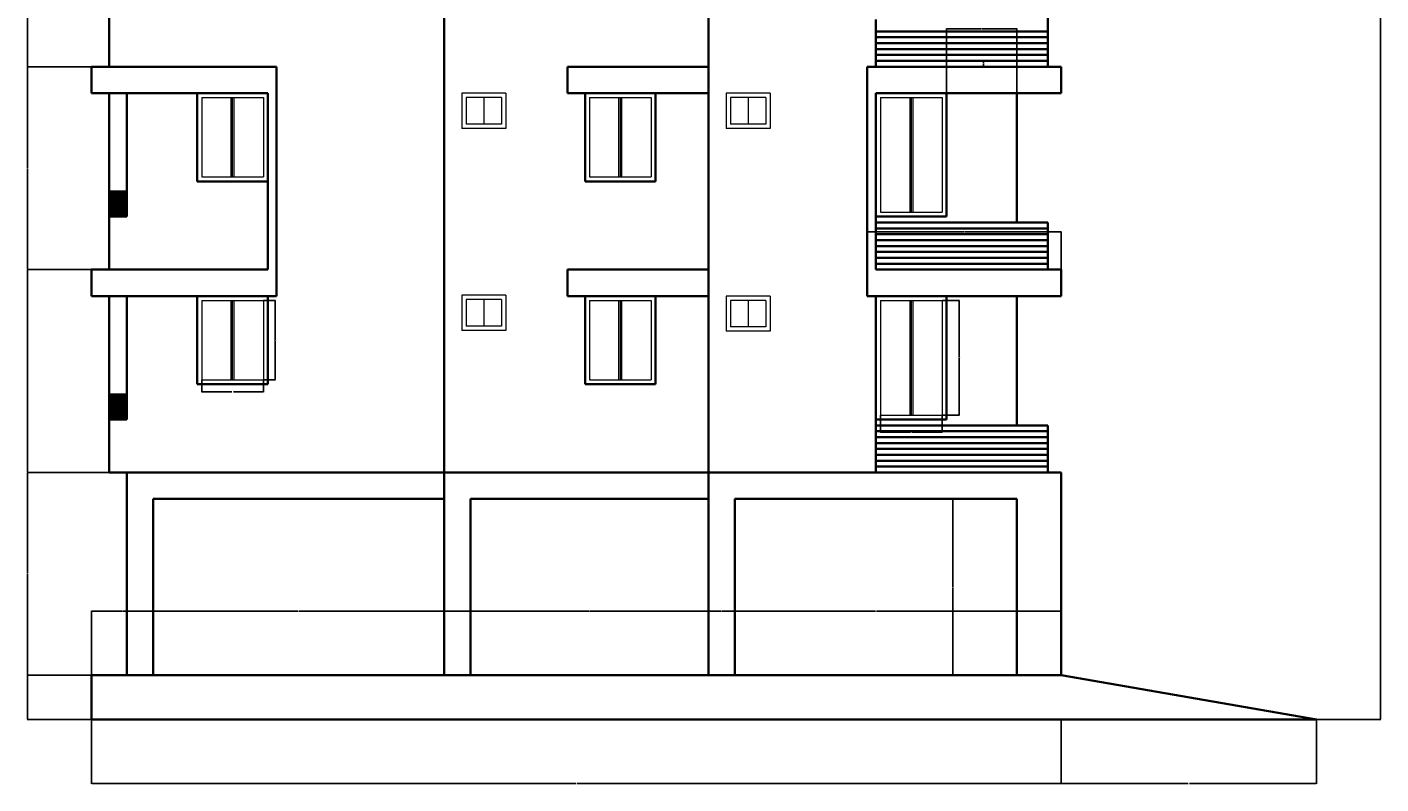
# Model space of a CAD drawing. Units: inches. Extents: x 2136 to 3058, y 322 to 1274.
# Tile 1 of 3: x 2136 to 3058, y 322 to 837. Entities that reach past the tile are written whole.
import ezdxf

# ---------------------------------------------------------------- set-up
doc = ezdxf.new("R2010")
doc.units = ezdxf.units.IN
for name, color, linetype, lineweight in [('A-ANNO-DIMS', 2, 'Continuous', 18), ('A-ELEV', 7, 'Continuous', 35), ('A-GLAZ', 4, 'Continuous', 18)]:
    doc.layers.add(name, color=color, linetype=linetype, lineweight=lineweight)
doc.styles.get("Standard").update_dxf_attribs({"font": 'arial.ttf'})
doc.dimstyles.get("Standard").update_dxf_attribs({"dimtxt": 0.18, "dimasz": 0.18, "dimexe": 0.18, "dimexo": 0.0625, "dimgap": 0.09, "dimtad": 0, "dimtih": 1, "dimtoh": 1, "dimdec": 4, "dimzin": 0, "dimdsep": 46, "dimtxsty": 'Standard', "dimcen": 0.09, "dimadec": 0, "dimazin": 0, "dimtfac": 1, "dimtdec": 4, "dimtofl": 0, "dimtmove": 0, "dimatfit": 3, "dimfxl": 1, "dimtolj": 1, "dimtzin": 0, "dimarcsym": 0})

# ---------------------------------------------------------------- blocks, each defined once
blk = doc.blocks.new('WIN-SMALL')
for p, q in [((2458.76, 1064.68), (2434.76, 1064.68)), ((2434.76, 1064.68), (2434.76, 1046.68)), ((2446.76, 1064.68), (2446.76, 1046.68)), ((2458.76, 1064.68), (2458.76, 1046.68)), ((2458.76, 1046.68), (2434.76, 1046.68))]:
    blk.add_line(p, q)
blk = doc.blocks.new('WIN-1200')
for p, q in [((2254.76, 650.67), (2254.76, 596.67)), ((2254.76, 650.67), (2296.76, 650.67)), ((2274.76, 596.67), (2274.76, 650.67)), ((2275.76, 596.67), (2275.76, 650.67)), ((2276.76, 596.67), (2276.76, 650.67)), ((2296.76, 650.67), (2296.76, 596.67)), ((2254.76, 596.67), (2296.76, 596.67))]:
    blk.add_line(p, q)
blk = doc.blocks.new('WIN-TALL')
for p, q in [((2716.76, 650.68), (2716.76, 572.68)), ((2716.76, 650.68), (2758.76, 650.68)), ((2736.76, 650.68), (2736.76, 572.68)), ((2737.76, 650.68), (2737.76, 572.68)), ((2738.76, 650.68), (2738.76, 572.68)), ((2758.76, 650.68), (2758.76, 572.68)), ((2716.76, 572.68), (2758.76, 572.68))]:
    blk.add_line(p, q)
blk = doc.blocks.new('*D6')
at = {"layer": 'A-ANNO-DIMS', "color": 0, "lineweight": -2, "transparency": 16777216}
for p, q in [((2296.82, 650.67), (2305.04, 650.67)), ((2304.86, 650.49), (2304.86, 623.86)), ((2304.86, 596.85), (2304.86, 623.49)), ((2296.82, 596.67), (2305.04, 596.67))]:
    blk.add_line(p, q, dxfattribs=at)
at = {"layer": 'A-ANNO-DIMS', "color": 0, "transparency": 16777216}
for points in [[(2304.83, 650.49), (2304.89, 650.49), (2304.86, 650.67)], [(2304.83, 596.85), (2304.89, 596.85), (2304.86, 596.67)]]:
    blk.add_solid(points, dxfattribs=at)
at = {"layer": 'Defpoints', "color": 0, "transparency": 16777216}
for p in [(2296.76, 650.67), (2304.86, 650.67), (2296.76, 596.67)]:
    blk.add_point(p, dxfattribs=at)
at = {"layer": 'A-ANNO-DIMS', "color": 0, "transparency": 16777216, "insert": (2304.86, 623.67), "char_height": 0.18, "attachment_point": 5}
blk.add_mtext('\\A1;WINDOW W1 54 TYP.', dxfattribs=at)
blk = doc.blocks.new('*D7')
at = {"layer": 'A-ANNO-DIMS', "color": 0, "lineweight": -2, "transparency": 16777216}
for p, q in [((2254.76, 596.61), (2254.76, 588.39)), ((2296.76, 596.61), (2296.76, 588.39)), ((2254.94, 588.57), (2275.23, 588.57)), ((2296.58, 588.57), (2276.29, 588.57))]:
    blk.add_line(p, q, dxfattribs=at)
at = {"layer": 'A-ANNO-DIMS', "color": 0, "transparency": 16777216}
for points in [[(2254.94, 588.6), (2254.94, 588.54), (2254.76, 588.57)], [(2296.58, 588.6), (2296.58, 588.54), (2296.76, 588.57)]]:
    blk.add_solid(points, dxfattribs=at)
at = {"layer": 'Defpoints', "color": 0, "transparency": 16777216}
for p in [(2254.76, 596.67), (2296.76, 596.67), (2296.76, 588.57)]:
    blk.add_point(p, dxfattribs=at)
at = {"layer": 'A-ANNO-DIMS', "color": 0, "transparency": 16777216, "insert": (2275.76, 588.57), "char_height": 0.18, "attachment_point": 5}
blk.add_mtext('\\A1;42 TYP.', dxfattribs=at)
blk = doc.blocks.new('*D8')
at = {"layer": 'A-ANNO-DIMS', "color": 0, "lineweight": -2, "transparency": 16777216}
for p, q in [((2758.82, 650.68), (2770.64, 650.68)), ((2770.46, 650.5), (2770.46, 611.87)), ((2770.46, 572.86), (2770.46, 611.5)), ((2758.82, 572.68), (2770.64, 572.68))]:
    blk.add_line(p, q, dxfattribs=at)
at = {"layer": 'A-ANNO-DIMS', "color": 0, "transparency": 16777216}
for points in [[(2770.43, 650.5), (2770.49, 650.5), (2770.46, 650.68)], [(2770.43, 572.86), (2770.49, 572.86), (2770.46, 572.68)]]:
    blk.add_solid(points, dxfattribs=at)
at = {"layer": 'Defpoints', "color": 0, "transparency": 16777216}
for p in [(2758.76, 650.68), (2770.46, 650.68), (2758.76, 572.68)]:
    blk.add_point(p, dxfattribs=at)
at = {"layer": 'A-ANNO-DIMS', "color": 0, "transparency": 16777216, "insert": (2770.46, 611.68), "char_height": 0.18, "attachment_point": 5}
blk.add_mtext('\\A1;FRENCH WINDOW W3 78 TYP.', dxfattribs=at)
blk = doc.blocks.new('*D9')
at = {"layer": 'A-ANNO-DIMS', "color": 0, "lineweight": -2, "transparency": 16777216}
for p, q in [((2716.76, 572.62), (2716.76, 560.8)), ((2758.76, 572.62), (2758.76, 560.8)), ((2716.94, 560.98), (2737.23, 560.98)), ((2758.58, 560.98), (2738.29, 560.98))]:
    blk.add_line(p, q, dxfattribs=at)
at = {"layer": 'A-ANNO-DIMS', "color": 0, "transparency": 16777216}
for points in [[(2716.94, 561.01), (2716.94, 560.95), (2716.76, 560.98)], [(2758.58, 561.01), (2758.58, 560.95), (2758.76, 560.98)]]:
    blk.add_solid(points, dxfattribs=at)
at = {"layer": 'Defpoints', "color": 0, "transparency": 16777216}
for p in [(2716.76, 572.68), (2758.76, 572.68), (2758.76, 560.98)]:
    blk.add_point(p, dxfattribs=at)
at = {"layer": 'A-ANNO-DIMS', "color": 0, "transparency": 16777216, "insert": (2737.76, 560.98), "char_height": 0.18, "attachment_point": 5}
blk.add_mtext('\\A1;42 TYP.', dxfattribs=at)
blk = doc.blocks.new('*D10')
at = {"layer": 'A-ANNO-DIMS', "color": 0, "lineweight": -2, "transparency": 16777216}
for p, q in [((2179.76, 365.62), (2179.76, 321.8)), ((2839.76, 365.62), (2839.76, 321.8)), ((2179.94, 321.98), (2509.47, 321.98)), ((2839.58, 321.98), (2510.05, 321.98))]:
    blk.add_line(p, q, dxfattribs=at)
at = {"layer": 'A-ANNO-DIMS', "color": 0, "transparency": 16777216}
for points in [[(2179.94, 322.01), (2179.94, 321.95), (2179.76, 321.98)], [(2839.58, 322.01), (2839.58, 321.95), (2839.76, 321.98)]]:
    blk.add_solid(points, dxfattribs=at)
at = {"layer": 'Defpoints', "color": 0, "transparency": 16777216}
for p in [(2179.76, 365.68), (2839.76, 365.68), (2839.76, 321.98)]:
    blk.add_point(p, dxfattribs=at)
at = {"layer": 'A-ANNO-DIMS', "color": 0, "transparency": 16777216, "insert": (2509.76, 321.98), "char_height": 0.18, "attachment_point": 5}
blk.add_mtext('\\A1;660', dxfattribs=at)
blk = doc.blocks.new('*D11')
at = {"layer": 'A-ANNO-DIMS', "color": 0, "lineweight": -2, "transparency": 16777216}
for p, q in [((2839.76, 365.62), (2839.76, 321.8)), ((3013.64, 365.62), (3013.64, 321.8)), ((2839.94, 321.98), (2926.24, 321.98)), ((3013.46, 321.98), (2927.16, 321.98))]:
    blk.add_line(p, q, dxfattribs=at)
at = {"layer": 'A-ANNO-DIMS', "color": 0, "transparency": 16777216}
for points in [[(2839.94, 322.01), (2839.94, 321.95), (2839.76, 321.98)], [(3013.46, 322.01), (3013.46, 321.95), (3013.64, 321.98)]]:
    blk.add_solid(points, dxfattribs=at)
at = {"layer": 'Defpoints', "color": 0, "transparency": 16777216}
for p in [(2839.76, 365.68), (3013.64, 365.68), (3013.64, 321.98)]:
    blk.add_point(p, dxfattribs=at)
at = {"layer": 'A-ANNO-DIMS', "color": 0, "transparency": 16777216, "insert": (2926.7, 321.98), "char_height": 0.18, "attachment_point": 5}
blk.add_mtext('\\A1;173.88', dxfattribs=at)
blk = doc.blocks.new('*D12')
at = {"layer": 'A-ANNO-DIMS', "color": 0, "lineweight": -2, "transparency": 16777216}
for p, q in [((2830.82, 1229.68), (3057.52, 1229.68)), ((3057.34, 1229.5), (3057.34, 797.87)), ((3057.34, 365.86), (3057.34, 797.5)), ((2839.82, 365.68), (3057.52, 365.68))]:
    blk.add_line(p, q, dxfattribs=at)
at = {"layer": 'A-ANNO-DIMS', "color": 0, "transparency": 16777216}
for points in [[(3057.31, 1229.5), (3057.37, 1229.5), (3057.34, 1229.68)], [(3057.31, 365.86), (3057.37, 365.86), (3057.34, 365.68)]]:
    blk.add_solid(points, dxfattribs=at)
at = {"layer": 'Defpoints', "color": 0, "transparency": 16777216}
for p in [(2830.76, 1229.68), (3057.34, 1229.68), (2839.76, 365.68)]:
    blk.add_point(p, dxfattribs=at)
at = {"layer": 'A-ANNO-DIMS', "color": 0, "transparency": 16777216, "insert": (3057.34, 797.68), "char_height": 0.18, "attachment_point": 5}
blk.add_mtext('\\A1;864', dxfattribs=at)
blk = doc.blocks.new('*D13')
at = {"layer": 'A-ANNO-DIMS', "color": 0, "lineweight": -2, "transparency": 16777216}
for p, q in [((2179.7, 395.68), (2135.88, 395.68)), ((2136.06, 395.5), (2136.06, 380.87)), ((2136.06, 365.86), (2136.06, 380.5)), ((2179.7, 365.68), (2135.88, 365.68))]:
    blk.add_line(p, q, dxfattribs=at)
at = {"layer": 'A-ANNO-DIMS', "color": 0, "transparency": 16777216}
for points in [[(2136.03, 395.5), (2136.09, 395.5), (2136.06, 395.68)], [(2136.03, 365.86), (2136.09, 365.86), (2136.06, 365.68)]]:
    blk.add_solid(points, dxfattribs=at)
at = {"layer": 'Defpoints', "color": 0, "transparency": 16777216}
for p in [(2136.06, 395.68), (2179.76, 395.68), (2179.76, 365.68)]:
    blk.add_point(p, dxfattribs=at)
at = {"layer": 'A-ANNO-DIMS', "color": 0, "transparency": 16777216, "insert": (2136.06, 380.68), "char_height": 0.18, "attachment_point": 5}
blk.add_mtext('\\A1;30', dxfattribs=at)
blk = doc.blocks.new('*D14')
at = {"layer": 'A-ANNO-DIMS', "color": 0, "lineweight": -2, "transparency": 16777216}
for p, q in [((2191.7, 533.68), (2135.88, 533.68)), ((2136.06, 533.5), (2136.06, 464.87)), ((2136.06, 395.86), (2136.06, 464.5)), ((2179.7, 395.68), (2135.88, 395.68))]:
    blk.add_line(p, q, dxfattribs=at)
at = {"layer": 'A-ANNO-DIMS', "color": 0, "transparency": 16777216}
for points in [[(2136.03, 533.5), (2136.09, 533.5), (2136.06, 533.68)], [(2136.03, 395.86), (2136.09, 395.86), (2136.06, 395.68)]]:
    blk.add_solid(points, dxfattribs=at)
at = {"layer": 'Defpoints', "color": 0, "transparency": 16777216}
for p in [(2136.06, 533.68), (2191.76, 533.68), (2179.76, 395.68)]:
    blk.add_point(p, dxfattribs=at)
at = {"layer": 'A-ANNO-DIMS', "color": 0, "transparency": 16777216, "insert": (2136.06, 464.68), "char_height": 0.18, "attachment_point": 5}
blk.add_mtext('\\A1;138', dxfattribs=at)
blk = doc.blocks.new('*D15')
at = {"layer": 'A-ANNO-DIMS', "color": 0, "lineweight": -2, "transparency": 16777216}
for p, q in [((2179.7, 671.68), (2135.88, 671.68)), ((2136.06, 671.5), (2136.06, 602.87)), ((2136.06, 533.86), (2136.06, 602.5)), ((2191.7, 533.68), (2135.88, 533.68))]:
    blk.add_line(p, q, dxfattribs=at)
at = {"layer": 'A-ANNO-DIMS', "color": 0, "transparency": 16777216}
for points in [[(2136.03, 671.5), (2136.09, 671.5), (2136.06, 671.68)], [(2136.03, 533.86), (2136.09, 533.86), (2136.06, 533.68)]]:
    blk.add_solid(points, dxfattribs=at)
at = {"layer": 'Defpoints', "color": 0, "transparency": 16777216}
for p in [(2136.06, 671.68), (2179.76, 671.68), (2191.76, 533.68)]:
    blk.add_point(p, dxfattribs=at)
at = {"layer": 'A-ANNO-DIMS', "color": 0, "transparency": 16777216, "insert": (2136.06, 602.68), "char_height": 0.18, "attachment_point": 5}
blk.add_mtext('\\A1;138', dxfattribs=at)
blk = doc.blocks.new('*D16')
at = {"layer": 'A-ANNO-DIMS', "color": 0, "lineweight": -2, "transparency": 16777216}
for p, q in [((2179.7, 809.68), (2135.88, 809.68)), ((2136.06, 809.5), (2136.06, 740.87)), ((2136.06, 671.86), (2136.06, 740.5)), ((2179.7, 671.68), (2135.88, 671.68))]:
    blk.add_line(p, q, dxfattribs=at)
at = {"layer": 'A-ANNO-DIMS', "color": 0, "transparency": 16777216}
for points in [[(2136.03, 809.5), (2136.09, 809.5), (2136.06, 809.68)], [(2136.03, 671.86), (2136.09, 671.86), (2136.06, 671.68)]]:
    blk.add_solid(points, dxfattribs=at)
at = {"layer": 'Defpoints', "color": 0, "transparency": 16777216}
for p in [(2136.06, 809.68), (2179.76, 809.68), (2179.76, 671.68)]:
    blk.add_point(p, dxfattribs=at)
at = {"layer": 'A-ANNO-DIMS', "color": 0, "transparency": 16777216, "insert": (2136.06, 740.68), "char_height": 0.18, "attachment_point": 5}
blk.add_mtext('\\A1;138', dxfattribs=at)
blk = doc.blocks.new('*D17')
at = {"layer": 'A-ANNO-DIMS', "color": 0, "lineweight": -2, "transparency": 16777216}
for p, q in [((2179.7, 947.68), (2135.88, 947.68)), ((2136.06, 947.5), (2136.06, 878.87)), ((2136.06, 809.86), (2136.06, 878.5)), ((2179.7, 809.68), (2135.88, 809.68))]:
    blk.add_line(p, q, dxfattribs=at)
at = {"layer": 'A-ANNO-DIMS', "color": 0, "transparency": 16777216}
for points in [[(2136.03, 947.5), (2136.09, 947.5), (2136.06, 947.68)], [(2136.03, 809.86), (2136.09, 809.86), (2136.06, 809.68)]]:
    blk.add_solid(points, dxfattribs=at)
at = {"layer": 'Defpoints', "color": 0, "transparency": 16777216}
for p in [(2136.06, 947.68), (2179.76, 947.68), (2179.76, 809.68)]:
    blk.add_point(p, dxfattribs=at)
at = {"layer": 'A-ANNO-DIMS', "color": 0, "transparency": 16777216, "insert": (2136.06, 878.68), "char_height": 0.18, "attachment_point": 5}
blk.add_mtext('\\A1;138', dxfattribs=at)
blk = doc.blocks.new('*D39')
at = {"layer": 'A-ANNO-DIMS', "color": 0, "lineweight": -2, "transparency": 16777216}
for p, q in [((2830.696807, 813.683656), (2786.879307, 813.683656)), ((2787.059307, 813.503656), (2787.059307, 811.863656)), ((2787.059307, 809.863656), (2787.059307, 811.503656)), ((2830.696807, 809.683656), (2786.879307, 809.683656))]:
    blk.add_line(p, q, dxfattribs=at)
at = {"layer": 'A-ANNO-DIMS', "color": 0, "transparency": 16777216}
for points in [[(2787.029307, 813.503656), (2787.089307, 813.503656), (2787.059307, 813.683656)], [(2787.029307, 809.863656), (2787.089307, 809.863656), (2787.059307, 809.683656)]]:
    blk.add_solid(points, dxfattribs=at)
at = {"layer": 'Defpoints', "color": 0, "transparency": 16777216}
for p in [(2787.059307, 813.683656), (2830.759307, 813.683656), (2830.759307, 809.683656)]:
    blk.add_point(p, dxfattribs=at)
at = {"layer": 'A-ANNO-DIMS', "color": 0, "transparency": 16777216, "insert": (2787.059307, 811.683656), "char_height": 0.18, "attachment_point": 5}
blk.add_mtext('\\A1;4', dxfattribs=at)
blk = doc.blocks.new('*D41')
at = {"layer": 'A-ANNO-DIMS', "color": 0, "lineweight": -2, "transparency": 16777216}
for p, q in [((2707.76, 653.75), (2707.76, 697.56)), ((2707.94, 697.38), (2773.48, 697.38)), ((2839.58, 697.38), (2774.04, 697.38)), ((2839.76, 653.75), (2839.76, 697.56))]:
    blk.add_line(p, q, dxfattribs=at)
at = {"layer": 'A-ANNO-DIMS', "color": 0, "transparency": 16777216}
for points in [[(2707.94, 697.41), (2707.94, 697.35), (2707.76, 697.38)], [(2839.58, 697.41), (2839.58, 697.35), (2839.76, 697.38)]]:
    blk.add_solid(points, dxfattribs=at)
at = {"layer": 'Defpoints', "color": 0, "transparency": 16777216}
for p in [(2839.76, 697.38), (2707.76, 653.68), (2839.76, 653.68)]:
    blk.add_point(p, dxfattribs=at)
at = {"layer": 'A-ANNO-DIMS', "color": 0, "transparency": 16777216, "insert": (2773.76, 697.38), "char_height": 0.18, "attachment_point": 5}
blk.add_mtext('\\A1;132', dxfattribs=at)
blk = doc.blocks.new('*D43')
at = {"layer": 'A-ANNO-DIMS', "color": 0, "lineweight": -2, "transparency": 16777216}
for p, q in [((2761.76, 791.75), (2761.76, 835.56)), ((2761.94, 835.38), (2785.54, 835.38)), ((2809.58, 835.38), (2785.98, 835.38)), ((2809.76, 791.75), (2809.76, 835.56))]:
    blk.add_line(p, q, dxfattribs=at)
at = {"layer": 'A-ANNO-DIMS', "color": 0, "transparency": 16777216}
for points in [[(2761.94, 835.41), (2761.94, 835.35), (2761.76, 835.38)], [(2809.58, 835.41), (2809.58, 835.35), (2809.76, 835.38)]]:
    blk.add_solid(points, dxfattribs=at)
at = {"layer": 'Defpoints', "color": 0, "transparency": 16777216}
for p in [(2809.76, 835.38), (2761.76, 791.68), (2809.76, 791.68)]:
    blk.add_point(p, dxfattribs=at)
at = {"layer": 'A-ANNO-DIMS', "color": 0, "transparency": 16777216, "insert": (2785.76, 835.38), "char_height": 0.18, "attachment_point": 5}
blk.add_mtext('\\A1;48', dxfattribs=at)
blk = doc.blocks.new('*D51')
at = {"layer": 'A-ANNO-DIMS', "color": 0, "lineweight": -2, "transparency": 16777216}
for p, q in [((2179.76, 395.75), (2179.76, 439.56)), ((2179.94, 439.38), (2200.54, 439.38)), ((2221.58, 439.38), (2200.98, 439.38)), ((2221.76, 395.75), (2221.76, 439.56))]:
    blk.add_line(p, q, dxfattribs=at)
at = {"layer": 'A-ANNO-DIMS', "color": 0, "transparency": 16777216}
for points in [[(2179.94, 439.41), (2179.94, 439.35), (2179.76, 439.38)], [(2221.58, 439.41), (2221.58, 439.35), (2221.76, 439.38)]]:
    blk.add_solid(points, dxfattribs=at)
at = {"layer": 'Defpoints', "color": 0, "transparency": 16777216}
for p in [(2221.76, 439.38), (2179.76, 395.68), (2221.76, 395.68)]:
    blk.add_point(p, dxfattribs=at)
at = {"layer": 'A-ANNO-DIMS', "color": 0, "transparency": 16777216, "insert": (2200.76, 439.38), "char_height": 0.18, "attachment_point": 5}
blk.add_mtext('\\A1;42', dxfattribs=at)
blk = doc.blocks.new('*D52')
at = {"layer": 'A-ANNO-DIMS', "color": 0, "lineweight": -2, "transparency": 16777216}
for p, q in [((2221.76, 395.75), (2221.76, 439.56)), ((2221.94, 439.38), (2320.48, 439.38)), ((2419.58, 439.38), (2321.04, 439.38)), ((2419.76, 395.75), (2419.76, 439.56))]:
    blk.add_line(p, q, dxfattribs=at)
at = {"layer": 'A-ANNO-DIMS', "color": 0, "transparency": 16777216}
for points in [[(2221.94, 439.41), (2221.94, 439.35), (2221.76, 439.38)], [(2419.58, 439.41), (2419.58, 439.35), (2419.76, 439.38)]]:
    blk.add_solid(points, dxfattribs=at)
at = {"layer": 'Defpoints', "color": 0, "transparency": 16777216}
for p in [(2419.76, 439.38), (2221.76, 395.68), (2419.76, 395.68)]:
    blk.add_point(p, dxfattribs=at)
at = {"layer": 'A-ANNO-DIMS', "color": 0, "transparency": 16777216, "insert": (2320.76, 439.38), "char_height": 0.18, "attachment_point": 5}
blk.add_mtext('\\A1;198', dxfattribs=at)
blk = doc.blocks.new('*D53')
at = {"layer": 'A-ANNO-DIMS', "color": 0, "lineweight": -2, "transparency": 16777216}
for p, q in [((2419.76, 395.75), (2419.76, 439.56)), ((2419.94, 439.38), (2428.55, 439.38)), ((2437.58, 439.38), (2428.97, 439.38)), ((2437.76, 395.75), (2437.76, 439.56))]:
    blk.add_line(p, q, dxfattribs=at)
at = {"layer": 'A-ANNO-DIMS', "color": 0, "transparency": 16777216}
for points in [[(2419.94, 439.41), (2419.94, 439.35), (2419.76, 439.38)], [(2437.58, 439.41), (2437.58, 439.35), (2437.76, 439.38)]]:
    blk.add_solid(points, dxfattribs=at)
at = {"layer": 'Defpoints', "color": 0, "transparency": 16777216}
for p in [(2437.76, 439.38), (2419.76, 395.68), (2437.76, 395.68)]:
    blk.add_point(p, dxfattribs=at)
at = {"layer": 'A-ANNO-DIMS', "color": 0, "transparency": 16777216, "insert": (2428.76, 439.38), "char_height": 0.18, "attachment_point": 5}
blk.add_mtext('\\A1;18', dxfattribs=at)
blk = doc.blocks.new('*D54')
at = {"layer": 'A-ANNO-DIMS', "color": 0, "lineweight": -2, "transparency": 16777216}
for p, q in [((2437.76, 395.75), (2437.76, 439.56)), ((2437.94, 439.38), (2518.48, 439.38)), ((2599.58, 439.38), (2519.04, 439.38)), ((2599.76, 395.75), (2599.76, 439.56))]:
    blk.add_line(p, q, dxfattribs=at)
at = {"layer": 'A-ANNO-DIMS', "color": 0, "transparency": 16777216}
for points in [[(2437.94, 439.41), (2437.94, 439.35), (2437.76, 439.38)], [(2599.58, 439.41), (2599.58, 439.35), (2599.76, 439.38)]]:
    blk.add_solid(points, dxfattribs=at)
at = {"layer": 'Defpoints', "color": 0, "transparency": 16777216}
for p in [(2599.76, 439.38), (2437.76, 395.68), (2599.76, 395.68)]:
    blk.add_point(p, dxfattribs=at)
at = {"layer": 'A-ANNO-DIMS', "color": 0, "transparency": 16777216, "insert": (2518.76, 439.38), "char_height": 0.18, "attachment_point": 5}
blk.add_mtext('\\A1;162', dxfattribs=at)
blk = doc.blocks.new('*D55')
at = {"layer": 'A-ANNO-DIMS', "color": 0, "lineweight": -2, "transparency": 16777216}
for p, q in [((2599.76, 395.75), (2599.76, 439.56)), ((2599.94, 439.38), (2608.55, 439.38)), ((2617.58, 439.38), (2608.97, 439.38)), ((2617.76, 395.75), (2617.76, 439.56))]:
    blk.add_line(p, q, dxfattribs=at)
at = {"layer": 'A-ANNO-DIMS', "color": 0, "transparency": 16777216}
for points in [[(2599.94, 439.41), (2599.94, 439.35), (2599.76, 439.38)], [(2617.58, 439.41), (2617.58, 439.35), (2617.76, 439.38)]]:
    blk.add_solid(points, dxfattribs=at)
at = {"layer": 'Defpoints', "color": 0, "transparency": 16777216}
for p in [(2617.76, 439.38), (2599.76, 395.68), (2617.76, 395.68)]:
    blk.add_point(p, dxfattribs=at)
at = {"layer": 'A-ANNO-DIMS', "color": 0, "transparency": 16777216, "insert": (2608.76, 439.38), "char_height": 0.18, "attachment_point": 5}
blk.add_mtext('\\A1;18', dxfattribs=at)
blk = doc.blocks.new('*D56')
at = {"layer": 'A-ANNO-DIMS', "color": 0, "lineweight": -2, "transparency": 16777216}
for p, q in [((2617.76, 395.75), (2617.76, 439.56)), ((2617.94, 439.38), (2713.48, 439.38)), ((2809.58, 439.38), (2714.04, 439.38)), ((2809.76, 395.75), (2809.76, 439.56))]:
    blk.add_line(p, q, dxfattribs=at)
at = {"layer": 'A-ANNO-DIMS', "color": 0, "transparency": 16777216}
for points in [[(2617.94, 439.41), (2617.94, 439.35), (2617.76, 439.38)], [(2809.58, 439.41), (2809.58, 439.35), (2809.76, 439.38)]]:
    blk.add_solid(points, dxfattribs=at)
at = {"layer": 'Defpoints', "color": 0, "transparency": 16777216}
for p in [(2809.76, 439.38), (2617.76, 395.68), (2809.76, 395.68)]:
    blk.add_point(p, dxfattribs=at)
at = {"layer": 'A-ANNO-DIMS', "color": 0, "transparency": 16777216, "insert": (2713.76, 439.38), "char_height": 0.18, "attachment_point": 5}
blk.add_mtext('\\A1;192', dxfattribs=at)
blk = doc.blocks.new('*D57')
at = {"layer": 'A-ANNO-DIMS', "color": 0, "lineweight": -2, "transparency": 16777216}
for p, q in [((2809.76, 395.75), (2809.76, 439.56)), ((2809.94, 439.38), (2824.54, 439.38)), ((2839.58, 439.38), (2824.98, 439.38)), ((2839.76, 395.75), (2839.76, 439.56))]:
    blk.add_line(p, q, dxfattribs=at)
at = {"layer": 'A-ANNO-DIMS', "color": 0, "transparency": 16777216}
for points in [[(2809.94, 439.41), (2809.94, 439.35), (2809.76, 439.38)], [(2839.58, 439.41), (2839.58, 439.35), (2839.76, 439.38)]]:
    blk.add_solid(points, dxfattribs=at)
at = {"layer": 'Defpoints', "color": 0, "transparency": 16777216}
for p in [(2839.76, 439.38), (2809.76, 395.68), (2839.76, 395.68)]:
    blk.add_point(p, dxfattribs=at)
at = {"layer": 'A-ANNO-DIMS', "color": 0, "transparency": 16777216, "insert": (2824.76, 439.38), "char_height": 0.18, "attachment_point": 5}
blk.add_mtext('\\A1;30', dxfattribs=at)
blk = doc.blocks.new('*D58')
at = {"layer": 'A-ANNO-DIMS', "color": 0, "lineweight": -2, "transparency": 16777216}
for p, q in [((2809.7, 515.68), (2765.88, 515.68)), ((2766.06, 515.5), (2766.06, 455.87)), ((2766.06, 395.86), (2766.06, 455.5)), ((2809.7, 395.68), (2765.88, 395.68))]:
    blk.add_line(p, q, dxfattribs=at)
at = {"layer": 'A-ANNO-DIMS', "color": 0, "transparency": 16777216}
for points in [[(2766.03, 515.5), (2766.09, 515.5), (2766.06, 515.68)], [(2766.03, 395.86), (2766.09, 395.86), (2766.06, 395.68)]]:
    blk.add_solid(points, dxfattribs=at)
at = {"layer": 'Defpoints', "color": 0, "transparency": 16777216}
for p in [(2766.06, 515.68), (2809.76, 515.68), (2809.76, 395.68)]:
    blk.add_point(p, dxfattribs=at)
at = {"layer": 'A-ANNO-DIMS', "color": 0, "transparency": 16777216, "insert": (2766.06, 455.68), "char_height": 0.18, "attachment_point": 5}
blk.add_mtext('\\A1;120', dxfattribs=at)

msp = doc.modelspace()

# ---------------------------------------------------------------- linework, layer by layer
at = {"layer": 'A-ELEV'}
for p, q in [((2419.759, 1127.684), (2419.759, 395.684)), ((2599.759, 1127.684), (2599.759, 395.684)), ((2191.759, 929.684), (2191.759, 809.684)), ((2713.759, 841.684), (2713.759, 809.684)), ((2830.759, 809.684), (2830.759, 845.684)), ((2713.759, 833.684), (2830.759, 833.684)), ((2713.759, 829.684), (2830.759, 829.684)), ((2713.759, 825.684), (2830.759, 825.684)), ((2713.759, 821.684), (2830.759, 821.684)), ((2713.759, 817.684), (2830.759, 817.684)), ((2713.759, 813.684), (2830.759, 813.684)), ((2179.759, 809.684), (2179.759, 791.684)), ((2179.759, 809.684), (2305.759, 809.684)), ((2305.759, 809.684), (2305.759, 653.684)), ((2503.759, 809.684), (2599.759, 809.684)), ((2503.759, 809.684), (2503.759, 791.684)), ((2707.759, 809.684), (2839.759, 809.684)), ((2707.759, 809.684), (2707.759, 653.684)), ((2839.759, 809.684), (2839.759, 791.684)), ((2179.759, 791.684), (2299.759, 791.684)), ((2191.759, 791.684), (2191.759, 671.684)), ((2203.759, 791.684), (2203.759, 707.684)), ((2251.759, 791.684), (2251.759, 731.684)), ((2299.759, 791.684), (2299.759, 671.684)), ((2503.759, 791.684), (2599.759, 791.684)), ((2515.759, 791.684), (2515.759, 731.684)), ((2563.759, 791.684), (2563.759, 731.684)), ((2713.759, 791.684), (2713.759, 671.684)), ((2713.759, 791.684), (2839.759, 791.684)), ((2761.759, 791.684), (2761.759, 707.684)), ((2809.759, 791.684), (2809.759, 703.684)), ((2251.759, 731.684), (2299.759, 731.684)), ((2515.759, 731.684), (2563.759, 731.684)), ((2191.759, 724.684), (2203.759, 724.684)), ((2191.759, 723.684), (2203.759, 723.684)), ((2191.759, 722.684), (2203.759, 722.684)), ((2191.759, 721.684), (2203.759, 721.684)), ((2191.759, 720.684), (2203.759, 720.684)), ((2191.759, 719.684), (2203.759, 719.684)), ((2191.759, 718.684), (2203.759, 718.684)), ((2191.759, 717.684), (2203.759, 717.684)), ((2191.759, 716.684), (2203.759, 716.684)), ((2191.759, 715.684), (2203.759, 715.684)), ((2191.759, 714.684), (2203.759, 714.684)), ((2191.759, 713.684), (2203.759, 713.684)), ((2191.759, 712.684), (2203.759, 712.684)), ((2191.759, 711.684), (2203.759, 711.684)), ((2191.759, 710.684), (2203.759, 710.684)), ((2191.759, 709.684), (2203.759, 709.684)), ((2191.759, 708.684), (2203.759, 708.684)), ((2191.759, 707.684), (2203.759, 707.684)), ((2713.759, 707.684), (2761.759, 707.684)), ((2713.759, 703.684), (2830.759, 703.684)), ((2830.759, 671.684), (2830.759, 703.684)), ((2713.759, 699.684), (2830.759, 699.684)), ((2713.759, 695.684), (2830.759, 695.684)), ((2713.759, 691.684), (2830.759, 691.684)), ((2713.759, 687.684), (2830.759, 687.684)), ((2713.759, 683.684), (2830.759, 683.684)), ((2713.759, 679.684), (2830.759, 679.684)), ((2713.759, 675.684), (2830.759, 675.684)), ((2179.759, 671.684), (2299.759, 671.684)), ((2179.759, 671.684), (2179.759, 653.684)), ((2503.759, 671.684), (2599.759, 671.684)), ((2503.759, 671.684), (2503.759, 653.684)), ((2713.759, 671.684), (2839.759, 671.684)), ((2839.759, 671.684), (2839.759, 653.684)), ((2179.759, 653.684), (2305.759, 653.684)), ((2191.759, 653.684), (2191.759, 533.684)), ((2203.759, 653.684), (2203.759, 569.684)), ((2251.759, 653.672), (2251.759, 593.672)), ((2299.759, 653.684), (2299.759, 593.672)), ((2503.759, 653.684), (2599.759, 653.684)), ((2515.759, 653.684), (2515.759, 593.684)), ((2563.759, 653.684), (2563.759, 593.684)), ((2707.759, 653.684), (2839.759, 653.684)), ((2713.759, 653.684), (2713.759, 533.684)), ((2761.759, 653.684), (2761.759, 569.684)), ((2809.759, 653.684), (2809.759, 565.684)), ((2251.759, 593.672), (2299.759, 593.672)), ((2515.759, 593.684), (2563.759, 593.684)), ((2191.759, 586.684), (2203.759, 586.684)), ((2191.759, 585.684), (2203.759, 585.684)), ((2191.759, 584.684), (2203.759, 584.684)), ((2191.759, 583.684), (2203.759, 583.684)), ((2191.759, 582.684), (2203.759, 582.684)), ((2191.759, 581.684), (2203.759, 581.684)), ((2191.759, 580.684), (2203.759, 580.684)), ((2191.759, 579.684), (2203.759, 579.684)), ((2191.759, 578.684), (2203.759, 578.684)), ((2191.759, 577.684), (2203.759, 577.684)), ((2191.759, 576.684), (2203.759, 576.684)), ((2191.759, 575.684), (2203.759, 575.684)), ((2191.759, 574.684), (2203.759, 574.684)), ((2191.759, 573.684), (2203.759, 573.684)), ((2191.759, 572.684), (2203.759, 572.684)), ((2191.759, 571.684), (2203.759, 571.684)), ((2191.759, 570.684), (2203.759, 570.684)), ((2191.759, 569.684), (2203.759, 569.684)), ((2713.759, 569.684), (2761.759, 569.684)), ((2713.759, 565.684), (2830.759, 565.684)), ((2830.759, 533.684), (2830.759, 565.684)), ((2713.759, 561.684), (2830.759, 561.684)), ((2713.759, 557.684), (2830.759, 557.684)), ((2713.759, 553.684), (2830.759, 553.684)), ((2713.759, 549.684), (2830.759, 549.684)), ((2713.759, 545.684), (2830.759, 545.684)), ((2713.759, 541.684), (2830.759, 541.684)), ((2713.759, 537.684), (2830.759, 537.684)), ((2191.759, 533.684), (2839.759, 533.684)), ((2203.759, 533.684), (2203.759, 395.684)), ((2839.759, 533.684), (2839.759, 395.684)), ((2221.759, 515.684), (2221.759, 395.684)), ((2221.759, 515.684), (2419.759, 515.684)), ((2437.759, 515.684), (2437.759, 395.684)), ((2437.759, 515.684), (2599.759, 515.684)), ((2617.759, 515.684), (2617.759, 395.684)), ((2617.759, 515.684), (2809.759, 515.684)), ((2809.759, 515.684), (2809.759, 395.684)), ((2179.759, 395.684), (2839.759, 395.684)), ((2179.759, 395.684), (2179.759, 365.684)), ((2839.759, 395.684), (3013.64, 365.684)), ((2179.759, 365.684), (2839.759, 365.684)), ((2203.759, 365.684), (2839.759, 365.684)), ((2839.759, 365.684), (3013.64, 365.684))]:
    msp.add_line(p, q, dxfattribs=at)
at = {"layer": 'A-GLAZ'}
for p, q in [((2461.759, 791.684), (2431.759, 791.684)), ((2431.759, 791.684), (2431.759, 767.684)), ((2461.759, 791.684), (2461.759, 767.684)), ((2641.759, 791.684), (2611.759, 791.684)), ((2611.759, 791.684), (2611.759, 767.684)), ((2641.759, 791.684), (2641.759, 767.684)), ((2461.759, 767.684), (2431.759, 767.684)), ((2641.759, 767.684), (2611.759, 767.684)), ((2461.759, 654.289), (2431.759, 654.289)), ((2431.759, 654.289), (2431.759, 630.289)), ((2461.759, 654.289), (2461.759, 630.289)), ((2641.759, 653.684), (2611.759, 653.684)), ((2611.759, 653.684), (2611.759, 629.684)), ((2641.759, 653.684), (2641.759, 629.684)), ((2461.759, 630.289), (2431.759, 630.289)), ((2641.759, 629.684), (2611.759, 629.684))]:
    msp.add_line(p, q, dxfattribs=at)

# ---------------------------------------------------------------- block references
for name, p in [('WIN-1200', (0, 138.011)), ('WIN-SMALL', (0, -276)), ('WIN-1200', (264, 138.011)), ('WIN-SMALL', (180, -276)), ('WIN-TALL', (0, 138)), ('WIN-1200', (0, 0)), ('WIN-SMALL', (0, -413.394)), ('WIN-1200', (264, 0.011)), ('WIN-SMALL', (180, -414)), ('WIN-TALL', (0, 0))]:
    msp.add_blockref(name, p, dxfattribs=at)

# ---------------------------------------------------------------- dimensions: what is measured, and where the dimension line sits
at = {"layer": 'A-ANNO-DIMS'}
for base, p1, p2, angle, picture, middle in [((3057.34, 1229.684), (2839.759, 365.684), (2830.759, 1229.684), 90, '*D12', (3057.34, 797.684)), ((2136.059, 947.684), (2179.759, 809.684), (2179.759, 947.684), 90, '*D17', (2136.059, 878.684)), ((2787.059, 813.684), (2830.759, 809.684), (2830.759, 813.684), 90, '*D39', (2787.059, 811.684)), ((2136.059, 809.684), (2179.759, 671.684), (2179.759, 809.684), 90, '*D16', (2136.059, 740.684)), ((2136.059, 671.684), (2191.759, 533.684), (2179.759, 671.684), 90, '*D15', (2136.059, 602.684)), ((2136.059, 533.684), (2179.759, 395.684), (2191.759, 533.684), 90, '*D14', (2136.059, 464.684)), ((2766.059, 515.684), (2809.759, 395.684), (2809.759, 515.684), 90, '*D58', (2766.059, 455.684)), ((2419.759, 439.384), (2221.759, 395.684), (2419.759, 395.684), 0, '*D52', (2320.759, 439.384)), ((2136.059, 395.684), (2179.759, 365.684), (2179.759, 395.684), 90, '*D13', (2136.059, 380.684))]:
    dim = msp.add_linear_dim(base=base, p1=p1, p2=p2, angle=angle, dimstyle='Standard', override={"dimdec": 0, "dimlfac": 1, "dimrnd": 0, "dimzin": 0, "dimdsep": 46, "dimlunit": 2}, dxfattribs=at)
    dim.commit()
    dim.dimension.update_dxf_attribs({"geometry": picture, "text_midpoint": middle})
for base, p1, p2, override, picture, middle in [((2809.759, 835.384), (2761.759, 791.684), (2809.759, 791.684), {"dimdec": 0, "dimlfac": 1, "dimrnd": 0, "dimzin": 0, "dimdsep": 46, "dimlunit": 2}, '*D43', (2785.759, 835.384)), ((2839.759, 697.384), (2707.759, 653.684), (2839.759, 653.684), {"dimdec": 0, "dimlfac": 1, "dimrnd": 0, "dimzin": 0, "dimdsep": 46, "dimlunit": 2}, '*D41', (2773.759, 697.384)), ((2221.759, 439.384), (2179.759, 395.684), (2221.759, 395.684), {"dimdec": 0, "dimlfac": 1, "dimrnd": 0, "dimzin": 0, "dimdsep": 46, "dimlunit": 2}, '*D51', (2200.759, 439.384)), ((2437.759, 439.384), (2419.759, 395.684), (2437.759, 395.684), {"dimdec": 0, "dimlfac": 1, "dimrnd": 0, "dimzin": 0, "dimdsep": 46, "dimlunit": 2}, '*D53', (2428.759, 439.384)), ((2599.759, 439.384), (2437.759, 395.684), (2599.759, 395.684), {"dimdec": 0, "dimlfac": 1, "dimrnd": 0, "dimzin": 0, "dimdsep": 46, "dimlunit": 2}, '*D54', (2518.759, 439.384)), ((2617.759, 439.384), (2599.759, 395.684), (2617.759, 395.684), {"dimdec": 0, "dimlfac": 1, "dimrnd": 0, "dimzin": 0, "dimdsep": 46, "dimlunit": 2}, '*D55', (2608.759, 439.384)), ((2809.759, 439.384), (2617.759, 395.684), (2809.759, 395.684), {"dimdec": 0, "dimlfac": 1, "dimrnd": 0, "dimzin": 0, "dimdsep": 46, "dimlunit": 2}, '*D56', (2713.759, 439.384)), ((2839.759, 439.384), (2809.759, 395.684), (2839.759, 395.684), {"dimdec": 0, "dimlfac": 1, "dimrnd": 0, "dimzin": 0, "dimdsep": 46, "dimlunit": 2}, '*D57', (2824.759, 439.384)), ((2839.759, 321.984), (2179.759, 365.684), (2839.759, 365.684), {"dimdec": 0, "dimlfac": 1, "dimrnd": 0, "dimzin": 0, "dimdsep": 46, "dimlunit": 2}, '*D10', (2509.759, 321.984)), ((3013.64, 321.984), (2839.759, 365.684), (3013.64, 365.684), {"dimdec": 2, "dimlfac": 1, "dimrnd": 0, "dimzin": 0, "dimdsep": 46, "dimlunit": 2}, '*D11', (2926.7, 321.984))]:
    dim = msp.add_linear_dim(base=base, p1=p1, p2=p2, dimstyle='Standard', override=override, dxfattribs=at)
    dim.commit()
    dim.dimension.update_dxf_attribs({"geometry": picture, "text_midpoint": middle})
for base, p1, p2, text, picture, middle in [((2304.859, 650.672), (2296.759, 596.672), (2296.759, 650.672), 'WINDOW W1 <> TYP.', '*D6', (2304.859, 623.672)), ((2770.459, 650.684), (2758.759, 572.684), (2758.759, 650.684), 'FRENCH WINDOW W3 <> TYP.', '*D8', (2770.459, 611.684))]:
    dim = msp.add_linear_dim(base=base, p1=p1, p2=p2, angle=90, text=text, dimstyle='Standard', override={"dimdec": 0, "dimlfac": 1, "dimrnd": 0, "dimzin": 0, "dimdsep": 46, "dimlunit": 2}, dxfattribs=at)
    dim.commit()
    dim.dimension.update_dxf_attribs({"geometry": picture, "text_midpoint": middle})
for base, p1, p2, picture, middle in [((2296.759, 588.572), (2254.759, 596.672), (2296.759, 596.672), '*D7', (2275.759, 588.572)), ((2758.759, 560.984), (2716.759, 572.684), (2758.759, 572.684), '*D9', (2737.759, 560.984))]:
    dim = msp.add_linear_dim(base=base, p1=p1, p2=p2, text='<> TYP.', dimstyle='Standard', override={"dimdec": 0, "dimlfac": 1, "dimrnd": 0, "dimzin": 0, "dimdsep": 46, "dimlunit": 2}, dxfattribs=at)
    dim.commit()
    dim.dimension.update_dxf_attribs({"geometry": picture, "text_midpoint": middle})

doc.saveas('drawing.dxf')
